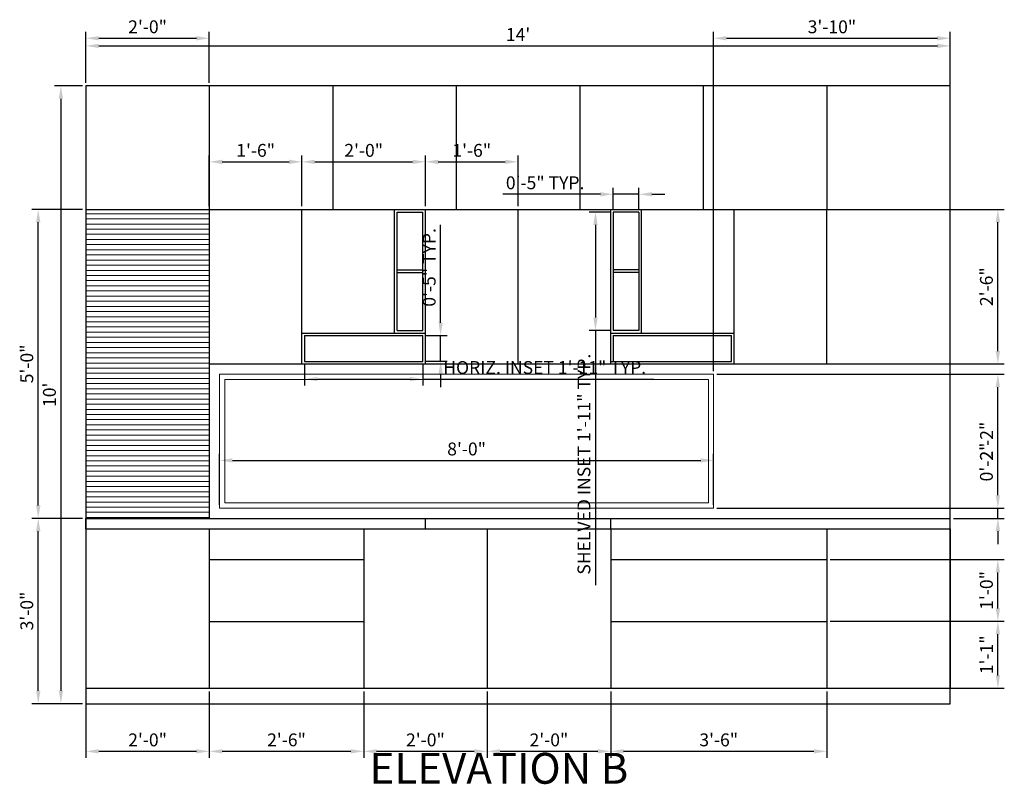
# Model space of a CAD drawing. Units: inches. Extents: x 125 to 951, y 142 to 358.
# Tile 3 of 4: x 538 to 730, y 207 to 356. Entities that reach past the tile are written whole.
import ezdxf

# ---------------------------------------------------------------- set-up
doc = ezdxf.new("R2010")
doc.units = ezdxf.units.IN
for name, color, linetype, lineweight in [('A-ANNO-DIMS', 2, 'Continuous', 18), ('A-ANNO-TEXT', 7, 'Continuous', 25), ('A-ELEV', 7, 'Continuous', 25), ('A-FLOR-CASE', 32, 'Continuous', 25), ('A-FLOR-CASE-PATT', 252, 'Continuous', 13), ('A-FLOR-CNTR', 30, 'Continuous', 25), ('A-GLAZ', 4, 'Continuous', 18)]:
    doc.layers.add(name, color=color, linetype=linetype, lineweight=lineweight)
doc.styles.get("Standard").update_dxf_attribs({"font": 'arial.ttf'})
doc.dimstyles.new('ISO-25', dxfattribs={"dimtxt": 2.5, "dimasz": 2.5, "dimexe": 1.25, "dimexo": 0.625, "dimtad": 1, "dimlunit": 3, "dimtxsty": 'Standard', "dimcen": 2.5, "dimadec": 0, "dimazin": 0, "dimtfac": 1, "dimtmove": 0, "dimatfit": 3, "dimfxl": 1, "dimarcsym": 0})

# ---------------------------------------------------------------- blocks, each defined once
blk = doc.blocks.new('*D5')
at = {"layer": 'A-ANNO-DIMS', "color": 0, "lineweight": -2, "transparency": 16777216}
for p, q in [((550.49, 342.83), (545.01, 342.83)), ((546.26, 340.33), (546.26, 225.33)), ((550.49, 222.83), (545.01, 222.83))]:
    blk.add_line(p, q, dxfattribs=at)
at = {"layer": 'A-ANNO-DIMS', "color": 0, "transparency": 16777216}
for points in [[(545.85, 340.33), (546.68, 340.33), (546.26, 342.83)], [(545.85, 225.33), (546.68, 225.33), (546.26, 222.83)]]:
    blk.add_solid(points, dxfattribs=at)
at = {"layer": 'Defpoints', "color": 0, "transparency": 16777216}
for p in [(551.11, 342.83), (546.26, 222.83), (551.11, 222.83)]:
    blk.add_point(p, dxfattribs=at)
at = {"layer": 'A-ANNO-DIMS', "color": 0, "transparency": 16777216, "insert": (544.36, 282.83), "char_height": 2.5, "attachment_point": 5, "rotation": 90}
blk.add_mtext("10'", dxfattribs=at)
blk = doc.blocks.new('*D6')
at = {"layer": 'A-ANNO-DIMS', "color": 0, "lineweight": -2, "transparency": 16777216}
for p, q in [((551.11, 343.45), (551.11, 351.85)), ((553.61, 350.6), (716.61, 350.6)), ((719.11, 343.45), (719.11, 351.85))]:
    blk.add_line(p, q, dxfattribs=at)
at = {"layer": 'A-ANNO-DIMS', "color": 0, "transparency": 16777216}
for points in [[(553.61, 351.01), (553.61, 350.18), (551.11, 350.6)], [(716.61, 351.01), (716.61, 350.18), (719.11, 350.6)]]:
    blk.add_solid(points, dxfattribs=at)
at = {"layer": 'Defpoints', "color": 0, "transparency": 16777216}
for p in [(719.11, 350.6), (551.11, 342.83), (719.11, 342.83)]:
    blk.add_point(p, dxfattribs=at)
at = {"layer": 'A-ANNO-DIMS', "color": 0, "transparency": 16777216, "insert": (635.11, 352.48), "char_height": 2.5, "attachment_point": 5}
blk.add_mtext("14'", dxfattribs=at)
blk = doc.blocks.new('CAB-INSET-HORIZ-23X5')
for p, q in [((0, 5), (23, 5)), ((0, 5), (0, 0)), ((23, 0), (23, 5)), ((0, 0), (23, 0))]:
    blk.add_line(p, q)
blk = doc.blocks.new('CAB-INSET-SHELVED-5X23')
for p, q in [((0, 0), (0, 23)), ((0, 23), (5, 23)), ((5, 0), (5, 23)), ((0, 11.75), (5, 11.75)), ((0, 11.25), (5, 11.25)), ((0, 0), (5, 0))]:
    blk.add_line(p, q)
blk = doc.blocks.new('*D17')
at = {"layer": 'A-ANNO-DIMS', "color": 0, "lineweight": -2, "transparency": 16777216}
for p, q in [((593.61, 288.7), (593.61, 284.63)), ((616.61, 288.7), (616.61, 284.63)), ((596.11, 285.88), (614.11, 285.88)), ((616.61, 285.88), (661.47, 285.88))]:
    blk.add_line(p, q, dxfattribs=at)
at = {"layer": 'A-ANNO-DIMS', "color": 0, "transparency": 16777216}
for points in [[(596.11, 286.29), (596.11, 285.46), (593.61, 285.88)], [(614.11, 286.29), (614.11, 285.46), (616.61, 285.88)]]:
    blk.add_solid(points, dxfattribs=at)
at = {"layer": 'Defpoints', "color": 0, "transparency": 16777216}
for p in [(593.61, 289.33), (616.61, 289.33), (616.61, 285.88)]:
    blk.add_point(p, dxfattribs=at)
at = {"layer": 'A-ANNO-DIMS', "color": 0, "transparency": 16777216, "insert": (640.29, 287.8), "char_height": 2.5, "attachment_point": 5}
blk.add_mtext('HORIZ. INSET 1\'-11" TYP.', dxfattribs=at)
blk = doc.blocks.new('*D18')
at = {"layer": 'A-ANNO-DIMS', "color": 0, "lineweight": -2, "transparency": 16777216}
for p, q in [((620.06, 296.83), (620.06, 315.82)), ((617.24, 294.33), (621.31, 294.33)), ((620.06, 289.33), (620.06, 294.33)), ((617.24, 289.33), (621.31, 289.33)), ((620.06, 286.83), (620.06, 284.33))]:
    blk.add_line(p, q, dxfattribs=at)
at = {"layer": 'A-ANNO-DIMS', "color": 0, "transparency": 16777216}
for points in [[(619.64, 296.83), (620.48, 296.83), (620.06, 294.33)], [(619.64, 286.83), (620.48, 286.83), (620.06, 289.33)]]:
    blk.add_solid(points, dxfattribs=at)
at = {"layer": 'Defpoints', "color": 0, "transparency": 16777216}
for p in [(616.61, 294.33), (620.06, 294.33), (616.61, 289.33)]:
    blk.add_point(p, dxfattribs=at)
at = {"layer": 'A-ANNO-DIMS', "color": 0, "transparency": 16777216, "insert": (618.16, 307.57), "char_height": 2.5, "attachment_point": 5, "rotation": 90}
blk.add_mtext('0\'-5" TYP.', dxfattribs=at)
blk = doc.blocks.new('*D19')
at = {"layer": 'A-ANNO-DIMS', "color": 0, "lineweight": -2, "transparency": 16777216}
for p, q in [((652.99, 318.33), (648.91, 318.33)), ((650.16, 315.83), (650.16, 297.83)), ((652.99, 295.33), (648.91, 295.33)), ((650.16, 295.33), (650.16, 245.88))]:
    blk.add_line(p, q, dxfattribs=at)
at = {"layer": 'A-ANNO-DIMS', "color": 0, "transparency": 16777216}
for points in [[(649.74, 315.83), (650.58, 315.83), (650.16, 318.33)], [(649.74, 297.83), (650.58, 297.83), (650.16, 295.33)]]:
    blk.add_solid(points, dxfattribs=at)
at = {"layer": 'Defpoints', "color": 0, "transparency": 16777216}
for p in [(653.61, 318.33), (650.16, 295.33), (653.61, 295.33)]:
    blk.add_point(p, dxfattribs=at)
at = {"layer": 'A-ANNO-DIMS', "color": 0, "transparency": 16777216, "insert": (648.24, 269.35), "char_height": 2.5, "attachment_point": 5, "rotation": 90}
blk.add_mtext('SHELVED INSET 1\'-11" TYP.', dxfattribs=at)
blk = doc.blocks.new('*D20')
at = {"layer": 'A-ANNO-DIMS', "color": 0, "lineweight": -2, "transparency": 16777216}
for p, q in [((651.11, 321.78), (632.12, 321.78)), ((653.61, 318.95), (653.61, 323.03)), ((658.61, 321.78), (653.61, 321.78)), ((658.61, 318.95), (658.61, 323.03)), ((661.11, 321.78), (663.61, 321.78))]:
    blk.add_line(p, q, dxfattribs=at)
at = {"layer": 'A-ANNO-DIMS', "color": 0, "transparency": 16777216}
for points in [[(651.11, 322.19), (651.11, 321.36), (653.61, 321.78)], [(661.11, 322.19), (661.11, 321.36), (658.61, 321.78)]]:
    blk.add_solid(points, dxfattribs=at)
at = {"layer": 'Defpoints', "color": 0, "transparency": 16777216}
for p in [(653.61, 321.78), (653.61, 318.33), (658.61, 318.33)]:
    blk.add_point(p, dxfattribs=at)
at = {"layer": 'A-ANNO-DIMS', "color": 0, "transparency": 16777216, "insert": (640.37, 323.68), "char_height": 2.5, "attachment_point": 5}
blk.add_mtext('0\'-5" TYP.', dxfattribs=at)
blk = doc.blocks.new('*D47')
at = {"layer": 'A-ANNO-DIMS', "color": 0, "lineweight": -2, "transparency": 16777216}
for p, q in [((551.11, 225.2), (551.11, 212.33)), ((575.11, 225.2), (575.11, 212.33)), ((553.61, 213.58), (572.61, 213.58))]:
    blk.add_line(p, q, dxfattribs=at)
at = {"layer": 'A-ANNO-DIMS', "color": 0, "transparency": 16777216}
for points in [[(553.61, 213.99), (553.61, 213.16), (551.11, 213.58)], [(572.61, 213.99), (572.61, 213.16), (575.11, 213.58)]]:
    blk.add_solid(points, dxfattribs=at)
at = {"layer": 'Defpoints', "color": 0, "transparency": 16777216}
for p in [(551.11, 225.83), (575.11, 225.83), (575.11, 213.58)]:
    blk.add_point(p, dxfattribs=at)
at = {"layer": 'A-ANNO-DIMS', "color": 0, "transparency": 16777216, "insert": (563.11, 215.48), "char_height": 2.5, "attachment_point": 5}
blk.add_mtext('2\'-0"', dxfattribs=at)
blk = doc.blocks.new('*D48')
at = {"layer": 'A-ANNO-DIMS', "color": 0, "lineweight": -2, "transparency": 16777216}
for p, q in [((575.11, 225.2), (575.11, 212.33)), ((605.11, 225.2), (605.11, 212.33)), ((577.61, 213.58), (602.61, 213.58))]:
    blk.add_line(p, q, dxfattribs=at)
at = {"layer": 'A-ANNO-DIMS', "color": 0, "transparency": 16777216}
for points in [[(577.61, 213.99), (577.61, 213.16), (575.11, 213.58)], [(602.61, 213.99), (602.61, 213.16), (605.11, 213.58)]]:
    blk.add_solid(points, dxfattribs=at)
at = {"layer": 'Defpoints', "color": 0, "transparency": 16777216}
for p in [(575.11, 225.83), (605.11, 225.83), (605.11, 213.58)]:
    blk.add_point(p, dxfattribs=at)
at = {"layer": 'A-ANNO-DIMS', "color": 0, "transparency": 16777216, "insert": (590.11, 215.48), "char_height": 2.5, "attachment_point": 5}
blk.add_mtext('2\'-6"', dxfattribs=at)
blk = doc.blocks.new('*D49')
at = {"layer": 'A-ANNO-DIMS', "color": 0, "lineweight": -2, "transparency": 16777216}
for p, q in [((605.11, 225.2), (605.11, 212.33)), ((629.11, 225.2), (629.11, 212.33)), ((607.61, 213.58), (626.61, 213.58))]:
    blk.add_line(p, q, dxfattribs=at)
at = {"layer": 'A-ANNO-DIMS', "color": 0, "transparency": 16777216}
for points in [[(607.61, 213.99), (607.61, 213.16), (605.11, 213.58)], [(626.61, 213.99), (626.61, 213.16), (629.11, 213.58)]]:
    blk.add_solid(points, dxfattribs=at)
at = {"layer": 'Defpoints', "color": 0, "transparency": 16777216}
for p in [(605.11, 225.83), (629.11, 225.83), (629.11, 213.58)]:
    blk.add_point(p, dxfattribs=at)
at = {"layer": 'A-ANNO-DIMS', "color": 0, "transparency": 16777216, "insert": (617.11, 215.48), "char_height": 2.5, "attachment_point": 5}
blk.add_mtext('2\'-0"', dxfattribs=at)
blk = doc.blocks.new('*D50')
at = {"layer": 'A-ANNO-DIMS', "color": 0, "lineweight": -2, "transparency": 16777216}
for p, q in [((629.11, 225.2), (629.11, 212.33)), ((653.11, 225.2), (653.11, 212.33)), ((631.61, 213.58), (650.61, 213.58))]:
    blk.add_line(p, q, dxfattribs=at)
at = {"layer": 'A-ANNO-DIMS', "color": 0, "transparency": 16777216}
for points in [[(631.61, 213.99), (631.61, 213.16), (629.11, 213.58)], [(650.61, 213.99), (650.61, 213.16), (653.11, 213.58)]]:
    blk.add_solid(points, dxfattribs=at)
at = {"layer": 'Defpoints', "color": 0, "transparency": 16777216}
for p in [(629.11, 225.83), (653.11, 225.83), (653.11, 213.58)]:
    blk.add_point(p, dxfattribs=at)
at = {"layer": 'A-ANNO-DIMS', "color": 0, "transparency": 16777216, "insert": (641.11, 215.48), "char_height": 2.5, "attachment_point": 5}
blk.add_mtext('2\'-0"', dxfattribs=at)
blk = doc.blocks.new('*D51')
at = {"layer": 'A-ANNO-DIMS', "color": 0, "lineweight": -2, "transparency": 16777216}
for p, q in [((653.11, 225.2), (653.11, 212.33)), ((695.11, 225.2), (695.11, 212.33)), ((655.61, 213.58), (692.61, 213.58))]:
    blk.add_line(p, q, dxfattribs=at)
at = {"layer": 'A-ANNO-DIMS', "color": 0, "transparency": 16777216}
for points in [[(655.61, 213.99), (655.61, 213.16), (653.11, 213.58)], [(692.61, 213.99), (692.61, 213.16), (695.11, 213.58)]]:
    blk.add_solid(points, dxfattribs=at)
at = {"layer": 'Defpoints', "color": 0, "transparency": 16777216}
for p in [(653.11, 225.83), (695.11, 225.83), (695.11, 213.58)]:
    blk.add_point(p, dxfattribs=at)
at = {"layer": 'A-ANNO-DIMS', "color": 0, "transparency": 16777216, "insert": (674.11, 215.48), "char_height": 2.5, "attachment_point": 5}
blk.add_mtext('3\'-6"', dxfattribs=at)
blk = doc.blocks.new('*D52')
at = {"layer": 'A-ANNO-DIMS', "color": 0, "lineweight": -2, "transparency": 16777216}
for p, q in [((577.11, 261.45), (577.11, 271.33)), ((579.61, 270.08), (670.61, 270.08)), ((673.11, 261.45), (673.11, 271.33))]:
    blk.add_line(p, q, dxfattribs=at)
at = {"layer": 'A-ANNO-DIMS', "color": 0, "transparency": 16777216}
for points in [[(579.61, 270.49), (579.61, 269.66), (577.11, 270.08)], [(670.61, 270.49), (670.61, 269.66), (673.11, 270.08)]]:
    blk.add_solid(points, dxfattribs=at)
at = {"layer": 'Defpoints', "color": 0, "transparency": 16777216}
for p in [(673.11, 270.08), (577.11, 260.83), (673.11, 260.83)]:
    blk.add_point(p, dxfattribs=at)
at = {"layer": 'A-ANNO-DIMS', "color": 0, "transparency": 16777216, "insert": (625.11, 271.98), "char_height": 2.5, "attachment_point": 5}
blk.add_mtext('8\'-0"', dxfattribs=at)
blk = doc.blocks.new('*D53')
at = {"layer": 'A-ANNO-DIMS', "color": 0, "lineweight": -2, "transparency": 16777216}
for p, q in [((550.49, 318.83), (540.61, 318.83)), ((541.86, 261.33), (541.86, 316.33)), ((550.49, 258.83), (540.61, 258.83))]:
    blk.add_line(p, q, dxfattribs=at)
at = {"layer": 'A-ANNO-DIMS', "color": 0, "transparency": 16777216}
for points in [[(541.44, 316.33), (542.28, 316.33), (541.86, 318.83)], [(541.44, 261.33), (542.28, 261.33), (541.86, 258.83)]]:
    blk.add_solid(points, dxfattribs=at)
at = {"layer": 'Defpoints', "color": 0, "transparency": 16777216}
for p in [(541.86, 318.83), (551.11, 318.83), (551.11, 258.83)]:
    blk.add_point(p, dxfattribs=at)
at = {"layer": 'A-ANNO-DIMS', "color": 0, "transparency": 16777216, "insert": (539.96, 288.83), "char_height": 2.5, "attachment_point": 5, "rotation": 90}
blk.add_mtext('5\'-0"', dxfattribs=at)
blk = doc.blocks.new('*D54')
at = {"layer": 'A-ANNO-DIMS', "color": 0, "lineweight": -2, "transparency": 16777216}
for p, q in [((550.49, 258.83), (540.61, 258.83)), ((541.86, 225.33), (541.86, 256.33)), ((550.49, 222.83), (540.61, 222.83))]:
    blk.add_line(p, q, dxfattribs=at)
at = {"layer": 'A-ANNO-DIMS', "color": 0, "transparency": 16777216}
for points in [[(541.44, 256.33), (542.28, 256.33), (541.86, 258.83)], [(541.44, 225.33), (542.28, 225.33), (541.86, 222.83)]]:
    blk.add_solid(points, dxfattribs=at)
at = {"layer": 'Defpoints', "color": 0, "transparency": 16777216}
for p in [(541.86, 258.83), (551.11, 258.83), (551.11, 222.83)]:
    blk.add_point(p, dxfattribs=at)
at = {"layer": 'A-ANNO-DIMS', "color": 0, "transparency": 16777216, "insert": (539.96, 240.83), "char_height": 2.5, "attachment_point": 5, "rotation": 90}
blk.add_mtext('3\'-0"', dxfattribs=at)
blk = doc.blocks.new('*D55')
at = {"layer": 'A-ANNO-DIMS', "color": 0, "lineweight": -2, "transparency": 16777216}
for p, q in [((695.74, 318.83), (729.61, 318.83)), ((728.36, 291.33), (728.36, 316.33)), ((695.74, 288.83), (729.61, 288.83))]:
    blk.add_line(p, q, dxfattribs=at)
at = {"layer": 'A-ANNO-DIMS', "color": 0, "transparency": 16777216}
for points in [[(727.94, 316.33), (728.78, 316.33), (728.36, 318.83)], [(727.94, 291.33), (728.78, 291.33), (728.36, 288.83)]]:
    blk.add_solid(points, dxfattribs=at)
at = {"layer": 'Defpoints', "color": 0, "transparency": 16777216}
for p in [(695.11, 318.83), (728.36, 318.83), (695.11, 288.83)]:
    blk.add_point(p, dxfattribs=at)
at = {"layer": 'A-ANNO-DIMS', "color": 0, "transparency": 16777216, "insert": (726.46, 303.83), "char_height": 2.5, "attachment_point": 5, "rotation": 90}
blk.add_mtext('2\'-6"', dxfattribs=at)
blk = doc.blocks.new('*D56')
at = {"layer": 'A-ANNO-DIMS', "color": 0, "lineweight": -2, "transparency": 16777216}
for p, q in [((673.74, 286.83), (729.61, 286.83)), ((728.36, 263.33), (728.36, 284.33)), ((673.74, 260.83), (729.61, 260.83))]:
    blk.add_line(p, q, dxfattribs=at)
at = {"layer": 'A-ANNO-DIMS', "color": 0, "transparency": 16777216}
for points in [[(727.94, 284.33), (728.78, 284.33), (728.36, 286.83)], [(727.94, 263.33), (728.78, 263.33), (728.36, 260.83)]]:
    blk.add_solid(points, dxfattribs=at)
at = {"layer": 'Defpoints', "color": 0, "transparency": 16777216}
for p in [(673.11, 286.83), (728.36, 286.83), (673.11, 260.83)]:
    blk.add_point(p, dxfattribs=at)
at = {"layer": 'A-ANNO-DIMS', "color": 0, "transparency": 16777216, "insert": (726.48, 273.83), "char_height": 2.5, "attachment_point": 5, "rotation": 90}
blk.add_mtext('2\'-2"', dxfattribs=at)
blk = doc.blocks.new('*D57')
at = {"layer": 'A-ANNO-DIMS', "color": 0, "lineweight": -2, "transparency": 16777216}
for p, q in [((695.74, 238.83), (729.61, 238.83)), ((728.36, 228.33), (728.36, 236.33)), ((695.74, 225.83), (729.61, 225.83))]:
    blk.add_line(p, q, dxfattribs=at)
at = {"layer": 'A-ANNO-DIMS', "color": 0, "transparency": 16777216}
for points in [[(727.94, 236.33), (728.78, 236.33), (728.36, 238.83)], [(727.94, 228.33), (728.78, 228.33), (728.36, 225.83)]]:
    blk.add_solid(points, dxfattribs=at)
at = {"layer": 'Defpoints', "color": 0, "transparency": 16777216}
for p in [(695.11, 238.83), (728.36, 238.83), (695.11, 225.83)]:
    blk.add_point(p, dxfattribs=at)
at = {"layer": 'A-ANNO-DIMS', "color": 0, "transparency": 16777216, "insert": (726.48, 232.33), "char_height": 2.5, "attachment_point": 5, "rotation": 90}
blk.add_mtext('1\'-1"', dxfattribs=at)
blk = doc.blocks.new('*D58')
at = {"layer": 'A-ANNO-DIMS', "color": 0, "lineweight": -2, "transparency": 16777216}
for p, q in [((695.74, 250.83), (729.61, 250.83)), ((728.36, 241.33), (728.36, 248.33)), ((695.74, 238.83), (729.61, 238.83))]:
    blk.add_line(p, q, dxfattribs=at)
at = {"layer": 'A-ANNO-DIMS', "color": 0, "transparency": 16777216}
for points in [[(727.94, 248.33), (728.78, 248.33), (728.36, 250.83)], [(727.94, 241.33), (728.78, 241.33), (728.36, 238.83)]]:
    blk.add_solid(points, dxfattribs=at)
at = {"layer": 'Defpoints', "color": 0, "transparency": 16777216}
for p in [(695.11, 250.83), (728.36, 250.83), (695.11, 238.83)]:
    blk.add_point(p, dxfattribs=at)
at = {"layer": 'A-ANNO-DIMS', "color": 0, "transparency": 16777216, "insert": (726.46, 244.83), "char_height": 2.5, "attachment_point": 5, "rotation": 90}
blk.add_mtext('1\'-0"', dxfattribs=at)
blk = doc.blocks.new('*D59')
at = {"layer": 'A-ANNO-DIMS', "color": 0, "lineweight": -2, "transparency": 16777216}
for p, q in [((551.11, 343.45), (551.11, 353.33)), ((575.11, 343.45), (575.11, 353.33)), ((553.61, 352.08), (572.61, 352.08))]:
    blk.add_line(p, q, dxfattribs=at)
at = {"layer": 'A-ANNO-DIMS', "color": 0, "transparency": 16777216}
for points in [[(553.61, 352.49), (553.61, 351.66), (551.11, 352.08)], [(572.61, 352.49), (572.61, 351.66), (575.11, 352.08)]]:
    blk.add_solid(points, dxfattribs=at)
at = {"layer": 'Defpoints', "color": 0, "transparency": 16777216}
for p in [(575.11, 352.08), (551.11, 342.83), (575.11, 342.83)]:
    blk.add_point(p, dxfattribs=at)
at = {"layer": 'A-ANNO-DIMS', "color": 0, "transparency": 16777216, "insert": (563.11, 353.98), "char_height": 2.5, "attachment_point": 5}
blk.add_mtext('2\'-0"', dxfattribs=at)
blk = doc.blocks.new('*D60')
at = {"layer": 'A-ANNO-DIMS', "color": 0, "lineweight": -2, "transparency": 16777216}
for p, q in [((575.11, 319.45), (575.11, 329.33)), ((593.11, 319.45), (593.11, 329.33)), ((577.61, 328.08), (590.61, 328.08))]:
    blk.add_line(p, q, dxfattribs=at)
at = {"layer": 'A-ANNO-DIMS', "color": 0, "transparency": 16777216}
for points in [[(577.61, 328.49), (577.61, 327.66), (575.11, 328.08)], [(590.61, 328.49), (590.61, 327.66), (593.11, 328.08)]]:
    blk.add_solid(points, dxfattribs=at)
at = {"layer": 'Defpoints', "color": 0, "transparency": 16777216}
for p in [(593.11, 328.08), (575.11, 318.83), (593.11, 318.83)]:
    blk.add_point(p, dxfattribs=at)
at = {"layer": 'A-ANNO-DIMS', "color": 0, "transparency": 16777216, "insert": (584.11, 329.98), "char_height": 2.5, "attachment_point": 5}
blk.add_mtext('1\'-6"', dxfattribs=at)
blk = doc.blocks.new('*D61')
at = {"layer": 'A-ANNO-DIMS', "color": 0, "lineweight": -2, "transparency": 16777216}
for p, q in [((593.11, 319.45), (593.11, 329.33)), ((617.11, 319.45), (617.11, 329.33)), ((595.61, 328.08), (614.61, 328.08))]:
    blk.add_line(p, q, dxfattribs=at)
at = {"layer": 'A-ANNO-DIMS', "color": 0, "transparency": 16777216}
for points in [[(595.61, 328.49), (595.61, 327.66), (593.11, 328.08)], [(614.61, 328.49), (614.61, 327.66), (617.11, 328.08)]]:
    blk.add_solid(points, dxfattribs=at)
at = {"layer": 'Defpoints', "color": 0, "transparency": 16777216}
for p in [(617.11, 328.08), (593.11, 318.83), (617.11, 318.83)]:
    blk.add_point(p, dxfattribs=at)
at = {"layer": 'A-ANNO-DIMS', "color": 0, "transparency": 16777216, "insert": (605.11, 329.98), "char_height": 2.5, "attachment_point": 5}
blk.add_mtext('2\'-0"', dxfattribs=at)
blk = doc.blocks.new('*D62')
at = {"layer": 'A-ANNO-DIMS', "color": 0, "lineweight": -2, "transparency": 16777216}
for p, q in [((617.11, 319.45), (617.11, 329.33)), ((635.11, 319.45), (635.11, 329.33)), ((619.61, 328.08), (632.61, 328.08))]:
    blk.add_line(p, q, dxfattribs=at)
at = {"layer": 'A-ANNO-DIMS', "color": 0, "transparency": 16777216}
for points in [[(619.61, 328.49), (619.61, 327.66), (617.11, 328.08)], [(632.61, 328.49), (632.61, 327.66), (635.11, 328.08)]]:
    blk.add_solid(points, dxfattribs=at)
at = {"layer": 'Defpoints', "color": 0, "transparency": 16777216}
for p in [(635.11, 328.08), (617.11, 318.83), (635.11, 318.83)]:
    blk.add_point(p, dxfattribs=at)
at = {"layer": 'A-ANNO-DIMS', "color": 0, "transparency": 16777216, "insert": (626.11, 329.98), "char_height": 2.5, "attachment_point": 5}
blk.add_mtext('1\'-6"', dxfattribs=at)
blk = doc.blocks.new('*D63')
at = {"layer": 'A-ANNO-DIMS', "color": 0, "lineweight": -2, "transparency": 16777216}
for p, q in [((673.11, 287.45), (673.11, 353.33)), ((719.11, 289.45), (719.11, 353.33)), ((675.61, 352.08), (716.61, 352.08))]:
    blk.add_line(p, q, dxfattribs=at)
at = {"layer": 'A-ANNO-DIMS', "color": 0, "transparency": 16777216}
for points in [[(675.61, 352.49), (675.61, 351.66), (673.11, 352.08)], [(716.61, 352.49), (716.61, 351.66), (719.11, 352.08)]]:
    blk.add_solid(points, dxfattribs=at)
at = {"layer": 'Defpoints', "color": 0, "transparency": 16777216}
for p in [(719.11, 352.08), (719.11, 288.83), (673.11, 286.83)]:
    blk.add_point(p, dxfattribs=at)
at = {"layer": 'A-ANNO-DIMS', "color": 0, "transparency": 16777216, "insert": (696.11, 353.98), "char_height": 2.5, "attachment_point": 5}
blk.add_mtext('3\'-10"', dxfattribs=at)
blk = doc.blocks.new('*D64')
at = {"layer": 'A-ANNO-DIMS', "color": 0, "lineweight": -2, "transparency": 16777216}
for p, q in [((728.36, 263.33), (728.36, 273.72)), ((673.74, 260.83), (729.61, 260.83)), ((728.36, 258.83), (728.36, 260.83)), ((719.74, 258.83), (729.61, 258.83)), ((728.36, 256.33), (728.36, 253.83))]:
    blk.add_line(p, q, dxfattribs=at)
at = {"layer": 'A-ANNO-DIMS', "color": 0, "transparency": 16777216}
for points in [[(727.94, 263.33), (728.78, 263.33), (728.36, 260.83)], [(727.94, 256.33), (728.78, 256.33), (728.36, 258.83)]]:
    blk.add_solid(points, dxfattribs=at)
at = {"layer": 'Defpoints', "color": 0, "transparency": 16777216}
for p in [(673.11, 260.83), (728.36, 260.83), (719.11, 258.83)]:
    blk.add_point(p, dxfattribs=at)
at = {"layer": 'A-ANNO-DIMS', "color": 0, "transparency": 16777216, "insert": (726.46, 269.77), "char_height": 2.5, "attachment_point": 5, "rotation": 90}
blk.add_mtext('0\'-2"', dxfattribs=at)

msp = doc.modelspace()

# ---------------------------------------------------------------- hatches: boundary and pattern name
at = {"layer": 'A-FLOR-CASE-PATT'}
h = msp.add_hatch(dxfattribs=at)
h.set_pattern_fill('ANSI31', color=256, scale=0.314961, angle=-45, style=0)
h.paths.add_polyline_path([(551.111, 258.827), (575.111, 258.827), (575.111, 318.827), (551.111, 318.827)])

# ---------------------------------------------------------------- linework, layer by layer
at = {"layer": 'A-ELEV'}
for p, q in [((551.111, 342.827), (551.111, 222.827)), ((719.111, 342.827), (551.111, 342.827)), ((719.111, 222.827), (719.111, 342.827)), ((551.111, 222.827), (719.111, 222.827))]:
    msp.add_line(p, q, dxfattribs=at)
at = {"layer": 'A-FLOR-CASE'}
for p, q in [((551.111, 342.827), (551.111, 258.827)), ((575.111, 342.827), (575.111, 258.827)), ((575.111, 342.827), (575.111, 318.827)), ((599.111, 342.827), (599.111, 318.827)), ((623.111, 342.827), (623.111, 318.827)), ((647.111, 342.827), (647.111, 318.827)), ((671.111, 342.827), (671.111, 318.827)), ((695.111, 342.827), (695.111, 318.827)), ((551.111, 318.827), (719.111, 318.827)), ((593.111, 288.827), (593.111, 318.827)), ((611.111, 294.827), (611.111, 318.827)), ((617.111, 288.827), (617.111, 318.827)), ((635.111, 288.827), (635.111, 318.827)), ((653.111, 288.827), (653.111, 318.827)), ((659.111, 294.827), (659.111, 318.827)), ((677.111, 288.827), (677.111, 318.827)), ((695.111, 288.827), (695.111, 318.827)), ((611.611, 307.077), (616.611, 307.077)), ((593.111, 294.827), (617.111, 294.827)), ((653.111, 294.827), (658.611, 294.827)), ((653.611, 294.827), (677.111, 294.827)), ((616.611, 289.327), (616.611, 294.327)), ((575.111, 288.827), (719.111, 288.827)), ((575.111, 288.827), (575.111, 258.827)), ((575.111, 288.827), (575.111, 258.827)), ((575.111, 256.827), (575.111, 225.827)), ((605.111, 256.827), (605.111, 225.827)), ((629.111, 256.827), (629.111, 225.827)), ((653.111, 256.827), (653.111, 225.827)), ((695.111, 256.827), (695.111, 225.827)), ((719.111, 256.827), (719.111, 225.827)), ((575.111, 250.827), (605.111, 250.827)), ((653.111, 250.827), (695.111, 250.827)), ((575.111, 238.827), (605.111, 238.827)), ((653.111, 238.827), (695.111, 238.827)), ((551.111, 225.827), (719.111, 225.827))]:
    msp.add_line(p, q, dxfattribs=at)
at = {"layer": 'A-FLOR-CNTR'}
for p, q in [((551.111, 258.827), (575.111, 258.827)), ((551.111, 256.827), (551.111, 258.827)), ((575.111, 258.827), (719.111, 258.827)), ((617.111, 256.827), (617.111, 258.827)), ((653.111, 256.827), (653.111, 258.827)), ((551.111, 256.827), (719.111, 256.827))]:
    msp.add_line(p, q, dxfattribs=at)
at = {"layer": 'A-GLAZ'}
for p, q in [((577.111, 286.827), (577.111, 260.827)), ((577.111, 286.827), (673.111, 286.827)), ((578.111, 285.827), (578.111, 261.827)), ((578.111, 285.827), (672.111, 285.827)), ((672.111, 285.827), (672.111, 261.827)), ((673.111, 286.827), (673.111, 260.827)), ((577.111, 260.827), (673.111, 260.827)), ((578.111, 261.827), (672.111, 261.827))]:
    msp.add_line(p, q, dxfattribs=at)

# ---------------------------------------------------------------- block references
at = {"layer": 'A-FLOR-CASE'}
for name, p in [('CAB-INSET-SHELVED-5X23', (611.611, 295.327)), ('CAB-INSET-HORIZ-23X5', (593.611, 289.327)), ('CAB-INSET-HORIZ-23X5', (653.611, 289.327))]:
    msp.add_blockref(name, p, dxfattribs=at)
at = {"layer": 'A-FLOR-CASE', "rotation": 180}
msp.add_blockref('CAB-INSET-SHELVED-5X23', (658.611, 318.326), dxfattribs=at)

# ---------------------------------------------------------------- texts
at = {"layer": 'A-ANNO-TEXT', "insert": (606.254, 213.283), "char_height": 6, "attachment_point": 1}
msp.add_mtext_dynamic_manual_height_columns('ELEVATION B', width=56.58494, gutter_width=12.5, heights=[0], dxfattribs=at)

# ---------------------------------------------------------------- dimensions: what is measured, and where the dimension line sits
at = {"layer": 'A-ANNO-DIMS'}
for base, p1, p2, override, picture, middle in [((575.111, 352.077), (551.111, 342.827), (575.111, 342.827), {"dimdec": 1, "dimlfac": 1, "dimrnd": 0, "dimzin": 1, "dimdsep": 46, "dimlunit": 4, "dimfrac": 2}, '*D59', (563.111, 353.978)), ((719.111, 350.597), (551.111, 342.827), (719.111, 342.827), {"dimclrd": 0, "dimclre": 0, "dimclrt": 0}, '*D6', (635.111, 352.477)), ((719.111, 352.077), (673.111, 286.827), (719.111, 288.827), {"dimdec": 1, "dimlfac": 1, "dimrnd": 0, "dimzin": 1, "dimdsep": 46, "dimlunit": 4, "dimfrac": 2}, '*D63', (696.111, 353.979)), ((593.111, 328.077), (575.111, 318.827), (593.111, 318.827), {"dimdec": 1, "dimlfac": 1, "dimrnd": 0, "dimzin": 1, "dimdsep": 46, "dimlunit": 4, "dimfrac": 2}, '*D60', (584.111, 329.978)), ((617.111, 328.077), (593.111, 318.827), (617.111, 318.827), {"dimdec": 1, "dimlfac": 1, "dimrnd": 0, "dimzin": 1, "dimdsep": 46, "dimlunit": 4, "dimfrac": 2}, '*D61', (605.111, 329.978)), ((635.111, 328.077), (617.111, 318.827), (635.111, 318.827), {"dimdec": 1, "dimlfac": 1, "dimrnd": 0, "dimzin": 1, "dimdsep": 46, "dimlunit": 4, "dimfrac": 2}, '*D62', (626.111, 329.978)), ((673.111, 270.077), (577.111, 260.827), (673.111, 260.827), {"dimdec": 1, "dimlfac": 1, "dimrnd": 0, "dimzin": 1, "dimdsep": 46, "dimlunit": 4, "dimfrac": 2}, '*D52', (625.111, 271.978)), ((575.111, 213.577), (551.111, 225.827), (575.111, 225.827), {"dimdec": 1, "dimlfac": 1, "dimrnd": 0, "dimzin": 1, "dimdsep": 46, "dimlunit": 4, "dimfrac": 2}, '*D47', (563.111, 215.478)), ((605.111, 213.577), (575.111, 225.827), (605.111, 225.827), {"dimdec": 1, "dimlfac": 1, "dimrnd": 0, "dimzin": 1, "dimdsep": 46, "dimlunit": 4, "dimfrac": 2}, '*D48', (590.111, 215.478)), ((629.111, 213.577), (605.111, 225.827), (629.111, 225.827), {"dimdec": 1, "dimlfac": 1, "dimrnd": 0, "dimzin": 1, "dimdsep": 46, "dimlunit": 4, "dimfrac": 2}, '*D49', (617.111, 215.478)), ((653.111, 213.577), (629.111, 225.827), (653.111, 225.827), {"dimdec": 1, "dimlfac": 1, "dimrnd": 0, "dimzin": 1, "dimdsep": 46, "dimlunit": 4, "dimfrac": 2}, '*D50', (641.111, 215.478)), ((695.111, 213.577), (653.111, 225.827), (695.111, 225.827), {"dimdec": 1, "dimlfac": 1, "dimrnd": 0, "dimzin": 1, "dimdsep": 46, "dimlunit": 4, "dimfrac": 2}, '*D51', (674.111, 215.479))]:
    dim = msp.add_linear_dim(base=base, p1=p1, p2=p2, dimstyle='ISO-25', override=override, dxfattribs=at)
    dim.commit()
    dim.dimension.update_dxf_attribs({"geometry": picture, "text_midpoint": middle})
for base, p1, p2, override, picture, middle in [((546.265, 222.827), (551.111, 342.827), (551.111, 222.827), {"dimclrd": 0, "dimclre": 0, "dimclrt": 0}, '*D5', (544.363, 282.827)), ((541.861, 318.827), (551.111, 258.827), (551.111, 318.827), {"dimdec": 1, "dimlfac": 1, "dimrnd": 0, "dimzin": 1, "dimdsep": 46, "dimlunit": 4, "dimfrac": 2}, '*D53', (539.96, 288.827)), ((728.361, 318.827), (695.111, 288.827), (695.111, 318.827), {"dimdec": 1, "dimlfac": 1, "dimrnd": 0, "dimzin": 1, "dimdsep": 46, "dimlunit": 4, "dimfrac": 2}, '*D55', (726.46, 303.827)), ((728.361, 286.827), (673.111, 260.827), (673.111, 286.827), {"dimdec": 1, "dimlfac": 1, "dimrnd": 0, "dimzin": 1, "dimdsep": 46, "dimlunit": 4, "dimfrac": 2}, '*D56', (726.481, 273.827)), ((728.361, 260.827), (719.111, 258.827), (673.111, 260.827), {"dimdec": 1, "dimlfac": 1, "dimrnd": 0, "dimzin": 1, "dimdsep": 46, "dimlunit": 4, "dimfrac": 2}, '*D64', (726.46, 269.775)), ((541.861, 258.827), (551.111, 222.827), (551.111, 258.827), {"dimdec": 1, "dimlfac": 1, "dimrnd": 0, "dimzin": 1, "dimdsep": 46, "dimlunit": 4, "dimfrac": 2}, '*D54', (539.959, 240.827)), ((728.361, 250.827), (695.111, 238.827), (695.111, 250.827), {"dimdec": 1, "dimlfac": 1, "dimrnd": 0, "dimzin": 1, "dimdsep": 46, "dimlunit": 4, "dimfrac": 2}, '*D58', (726.46, 244.827)), ((728.361, 238.827), (695.111, 225.827), (695.111, 238.827), {"dimdec": 1, "dimlfac": 1, "dimrnd": 0, "dimzin": 1, "dimdsep": 46, "dimlunit": 4, "dimfrac": 2}, '*D57', (726.481, 232.327))]:
    dim = msp.add_linear_dim(base=base, p1=p1, p2=p2, angle=90, dimstyle='ISO-25', override=override, dxfattribs=at)
    dim.commit()
    dim.dimension.update_dxf_attribs({"geometry": picture, "text_midpoint": middle})
for base, p1, p2, angle, text, picture, middle in [((653.611, 321.777), (658.611, 318.327), (653.611, 318.327), 180, '<> TYP.', '*D20', (640.367, 323.678)), ((650.161, 295.327), (653.611, 318.327), (653.611, 295.327), 270, 'SHELVED INSET <> TYP.', '*D19', (648.243, 269.352)), ((620.061, 294.327), (616.611, 289.327), (616.611, 294.327), 90, '<> TYP.', '*D18', (618.16, 307.571))]:
    dim = msp.add_linear_dim(base=base, p1=p1, p2=p2, angle=angle, text=text, dimstyle='ISO-25', override={"dimdec": 1, "dimlfac": 1, "dimrnd": 0, "dimzin": 1, "dimdsep": 46, "dimlunit": 4, "dimfrac": 2}, dxfattribs=at)
    dim.commit()
    dim.dimension.update_dxf_attribs({"geometry": picture, "text_midpoint": middle})
dim = msp.add_linear_dim(base=(616.611, 285.877), p1=(593.611, 289.327), p2=(616.611, 289.327), text='HORIZ. INSET <> TYP.', dimstyle='ISO-25', override={"dimdec": 1, "dimlfac": 1, "dimrnd": 0, "dimzin": 1, "dimdsep": 46, "dimlunit": 4, "dimfrac": 2}, dxfattribs=at)
dim.commit()
dim.dimension.update_dxf_attribs({"geometry": '*D17', "text_midpoint": (640.289, 287.795)})

doc.saveas('drawing.dxf')
